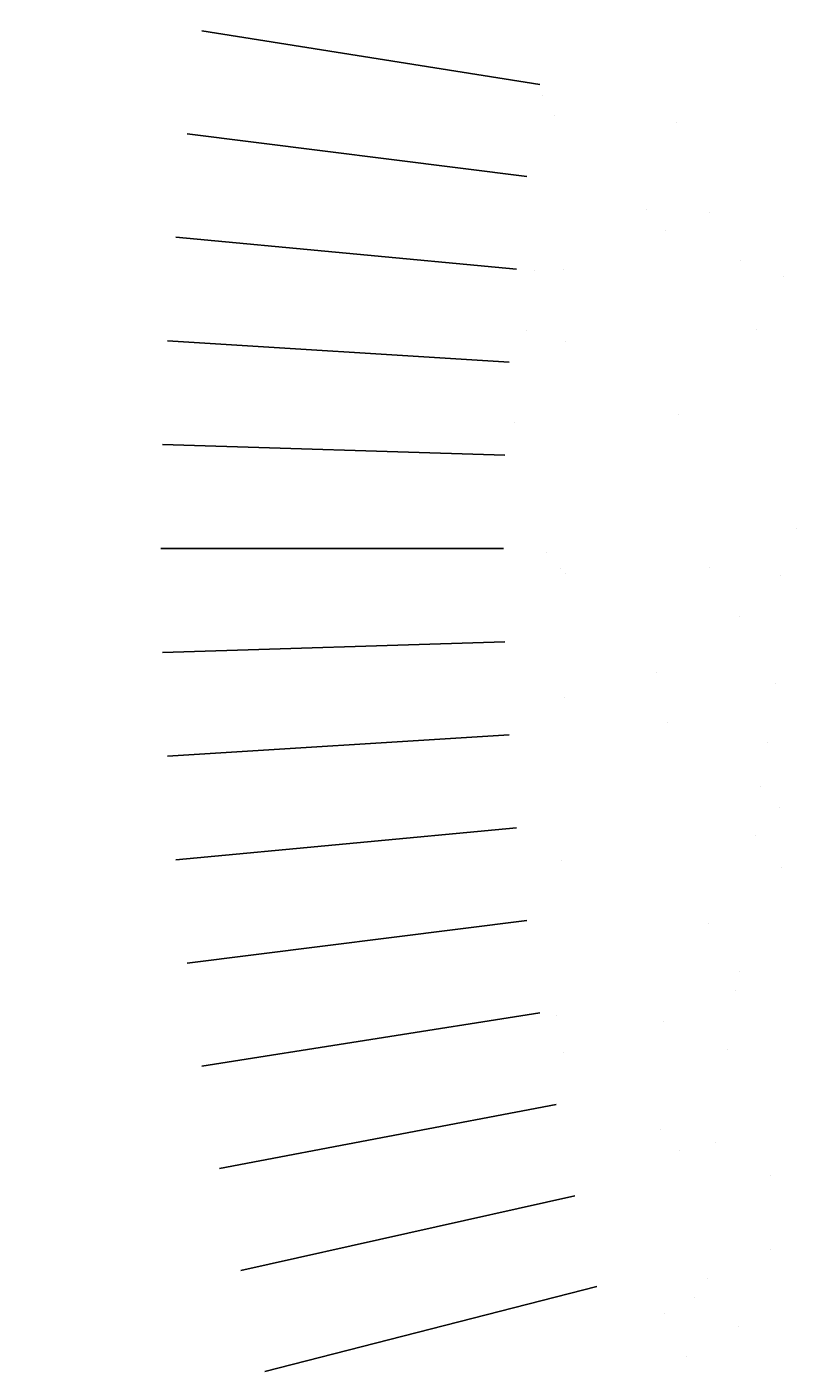
# Model space of a CAD drawing. Units: millimetres. Extents: x -857 to 54106, y -13666 to 13947.
# Tile 33 of 41: x 30856 to 31161, y 9453 to 9986. Entities that reach past the tile are written whole.
import ezdxf

# ---------------------------------------------------------------- set-up
doc = ezdxf.new("R2010")
doc.units = ezdxf.units.MM
doc.layers.add('A-ANNO-DIMS', color=2, linetype='Continuous', lineweight=18)
doc.layers.add('A-FURN', color=21, linetype='Continuous', lineweight=18)
doc.layers.add('A-HT', color=15, linetype='Continuous')
doc.styles.get("Standard").update_dxf_attribs({"font": 'arial.ttf'})
doc.dimstyles.new('ISO-25', dxfattribs={"dimtxt": 2.5, "dimasz": 2.5, "dimexe": 1.25, "dimexo": 0.625, "dimtad": 1, "dimtxsty": 'Standard', "dimcen": 2.5, "dimadec": 0, "dimazin": 0, "dimtfac": 1, "dimtmove": 0, "dimatfit": 3, "dimfxl": 1, "dimarcsym": 0})

# ---------------------------------------------------------------- blocks, each defined once
blk = doc.blocks.new('*X18')
at = {"color": 0}
for p, q in [((1.94501, 2.84522), (1.94501, 2.84522)), ((1.90437, 2.83986), (1.90437, 2.83986)), ((1.80172, 2.83302), (1.80172, 2.83302)), ((1.87834, 2.83644), (1.87834, 2.83644)), ((2.0018, 2.8313), (2.0018, 2.8313)), ((1.81043, 2.8275), (1.81043, 2.8275)), ((2.00868, 2.82517), (2.00868, 2.82517)), ((2.20482, 2.82688), (2.20482, 2.82688)), ((1.8778, 2.8235), (1.8778, 2.8235)), ((1.90945, 2.82302), (1.90945, 2.82302)), ((2.01101, 2.82286), (2.01101, 2.82286)), ((2.06515, 2.8233), (2.06515, 2.8233)), ((2.13659, 2.82456), (2.13659, 2.82456)), ((2.22086, 2.82359), (2.22086, 2.82359)), ((1.85149, 2.78742), (1.85149, 2.78742)), ((1.86071, 2.77898), (1.86071, 2.77898)), ((2.05451, 2.783), (2.05451, 2.783)), ((2.07629, 2.77829), (2.07629, 2.77829)), ((2.20717, 2.77996), (2.20717, 2.77996)), ((2.25458, 2.78128), (2.25458, 2.78128)), ((2.33508, 2.77935), (2.33508, 2.77935)), ((1.81334, 2.77404), (1.81334, 2.77404)), ((1.94125, 2.77343), (1.94125, 2.77343)), ((2.2638, 2.77284), (2.2638, 2.77284)), ((2.32821, 2.76621), (2.32821, 2.76621)), ((2.35423, 2.76963), (2.35423, 2.76963)), ((2.31996, 2.76045), (2.31996, 2.76045)), ((1.85284, 2.75961), (1.85284, 2.75961)), ((2.00854, 2.75989), (2.00854, 2.75989)), ((2.16425, 2.76017), (2.16425, 2.76017)), ((2.26029, 2.75727), (2.26029, 2.75727)), ((2.21964, 2.75191), (2.21964, 2.75191)), ((1.87392, 2.74617), (1.87392, 2.74617)), ((2.02963, 2.74646), (2.02963, 2.74646)), ((2.18534, 2.74674), (2.18534, 2.74674)), ((2.19362, 2.74849), (2.19362, 2.74849)), ((2.34104, 2.74702), (2.34104, 2.74702)), ((1.90421, 2.73912), (1.90421, 2.73912)), ((2.10428, 2.7374), (2.10428, 2.7374)), ((2.1257, 2.73955), (2.1257, 2.73955)), ((2.08505, 2.7342), (2.08505, 2.7342)), ((2.27478, 2.73308), (2.27478, 2.73308)), ((2.3073, 2.73298), (2.3073, 2.73298)), ((1.88095, 2.72716), (1.88095, 2.72716)), ((2.01183, 2.72883), (2.01183, 2.72883)), ((2.05903, 2.73077), (2.05903, 2.73077)), ((2.11349, 2.72895), (2.11349, 2.72895)), ((2.13974, 2.72822), (2.13974, 2.72822)), ((1.99111, 2.72183), (1.99111, 2.72183))]:
    blk.add_line(p, q, dxfattribs=at)
blk = doc.blocks.new('A$C6796526C')
at = {"layer": 'A-HT'}
for p, q in [((1.7733, 0.19084), (1.8106, 0.04555)), ((1.73359, 0.18131), (1.76631, 0.03492)), ((1.6936, 0.17303), (1.7217, 0.02568)), ((1.24664, 0.16601), (1.22317, 0.01785)), ((1.65337, 0.16601), (1.67683, 0.01785)), ((1.28707, 0.16025), (1.26827, 0.01143)), ((1.61293, 0.16025), (1.63173, 0.01143)), ((1.32766, 0.15577), (1.31354, 0.00644)), ((1.57234, 0.15577), (1.58646, 0.00644)), ((1.36837, 0.15257), (1.35895, 0.00286)), ((1.40917, 0.15064), (1.40445, 0.00072)), ((1.45, 0.15), (1.45, 0)), ((1.49083, 0.15064), (1.49555, 0.00072)), ((1.53163, 0.15257), (1.54105, 0.00286))]:
    blk.add_line(p, q, dxfattribs=at)
at = {"layer": 'A-HT', "extrusion": (0, 0, -1), "zscale": -1, "rotation": 180}
blk.add_blockref('*X18', (0.55, 3), dxfattribs=at)
blk = doc.blocks.new('*D48')
at = {"layer": 'A-ANNO-DIMS', "color": 0, "lineweight": -2, "transparency": 16777216}
for p, q in [((30908.63, 11089.46), (30501.38, 11089.46)), ((30502.63, 11086.96), (30502.63, 8471.5)), ((30908.63, 8469), (30501.38, 8469))]:
    blk.add_line(p, q, dxfattribs=at)
at = {"layer": 'A-ANNO-DIMS', "color": 0, "transparency": 16777216}
for points in [[(30502.21, 11086.96), (30503.05, 11086.96), (30502.63, 11089.46)], [(30502.21, 8471.5), (30503.05, 8471.5), (30502.63, 8469)]]:
    blk.add_solid(points, dxfattribs=at)
at = {"layer": 'Defpoints', "color": 0, "transparency": 16777216}
for p in [(30909.25, 11089.46), (30502.63, 8469), (30909.25, 8469)]:
    blk.add_point(p, dxfattribs=at)
at = {"layer": 'A-ANNO-DIMS', "color": 0, "transparency": 16777216, "insert": (30500.73, 9779.23), "char_height": 2.5, "attachment_point": 5, "rotation": 90}
blk.add_mtext('2620 TYP.', dxfattribs=at)

msp = doc.modelspace()

# ---------------------------------------------------------------- block references
at = {"layer": 'A-FURN', "xscale": 903.6084929786902, "yscale": 903.6084929786902, "zscale": 903.6084929786902, "rotation": 269.9999999999988}
msp.add_blockref('A$C6796526C', (30909.253, 11089.463), dxfattribs=at)

# ---------------------------------------------------------------- dimensions: what is measured, and where the dimension line sits
at = {"layer": 'A-ANNO-DIMS'}
dim = msp.add_linear_dim(base=(30502.63, 8468.999), p1=(30909.254, 11089.463), p2=(30909.254, 8468.999), angle=270, text='<> TYP.', dimstyle='ISO-25', override={"dimdec": 0, "dimrnd": 0, "dimzin": 0, "dimlunit": 2}, dxfattribs=at)
dim.commit()
dim.dimension.update_dxf_attribs({"geometry": '*D48', "text_midpoint": (30500.728, 9779.231)})

doc.saveas('drawing.dxf')
